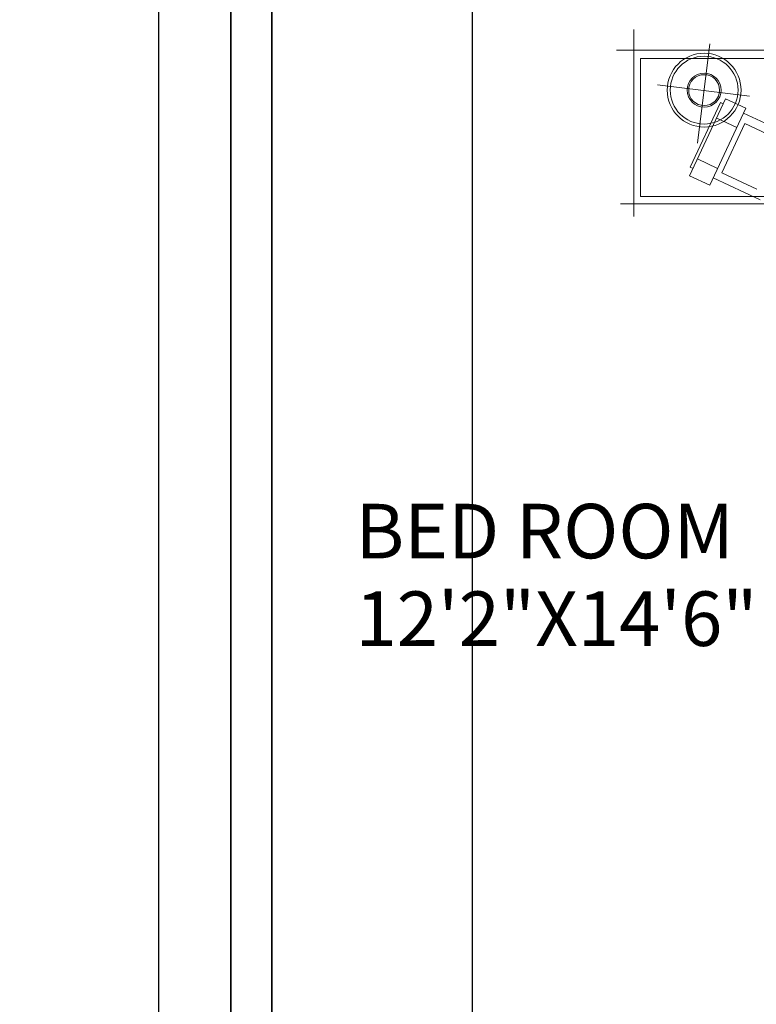
# Model space of a CAD drawing. Units: inches. Extents: x -438 to 102, y -60 to 1091.
# Tile 15 of 20: x -149 to -68, y 699 to 807. Entities that reach past the tile are written whole.
import ezdxf

# ---------------------------------------------------------------- set-up
doc = ezdxf.new("R2010")
doc.units = ezdxf.units.IN
doc.header["$MEASUREMENT"] = 0
doc.layers.add('A-ANNO-DIMS', color=217, linetype='Continuous', lineweight=18, true_color=0x93278f)
doc.layers.add('A-WALL', color=2, linetype='Continuous', lineweight=35, true_color=0xf1eb1f)
doc.layers.add('A-AREA-IDEN', color=4, linetype='Continuous', lineweight=18)
doc.layers.add('Furniture', color=7, linetype='Continuous', lineweight=15)
doc.styles.get("Standard").update_dxf_attribs({"font": 'arial.ttf'})
doc.dimstyles.get("Standard").update_dxf_attribs({"dimtxt": 8, "dimasz": 0.18, "dimexe": 0.18, "dimexo": 0.0625, "dimgap": 0.09, "dimtad": 0, "dimtih": 1, "dimtoh": 1, "dimdec": 4, "dimzin": 0, "dimdsep": 46, "dimlunit": 3, "dimtxsty": 'Standard', "dimcen": 0.09, "dimadec": 0, "dimazin": 0, "dimtfac": 1, "dimtdec": 4, "dimtofl": 0, "dimtmove": 0, "dimatfit": 3, "dimfxl": 1, "dimtolj": 1, "dimtzin": 0, "dimarcsym": 0})

# ---------------------------------------------------------------- blocks, each defined once
blk = doc.blocks.new('BED-DOUBLE-WITH-NIGHTSTANDS')
for p, q in [((-50.06, 0), (-50.06, -20.6)), ((-41.72, -1.6), (-43.05, -12.53)), ((-28.76, -2.28), (-51.98, -2.28)), ((-31.1, -3.21), (-49.32, -3.21)), ((-49.32, -3.21), (-49.32, -18.39)), ((-37.32, -7.35), (-47.47, -6.1)), ((-43.93, -16.11), (-39.96, -7.63)), ((-40.53, -8.03), (-43.86, -15.16)), ((-37.75, -8.67), (-41.72, -17.15)), ((-40.22, -8.18), (-40.53, -8.03)), ((-39.96, -7.63), (-37.75, -8.67)), ((-32.84, -11.63), (-38.01, -9.21)), ((-38.74, -10.79), (-40.95, -9.75)), ((-37.86, -10.36), (-40.39, -15.77)), ((-34, -12.16), (-37.86, -10.36)), ((-43.86, -15.16), (-43.55, -15.31)), ((-40.85, -15.29), (-43.06, -14.25)), ((-41.72, -17.15), (-43.93, -16.11)), ((-40.39, -15.77), (-36.53, -17.57)), ((-41.34, -16.34), (-36.18, -18.76)), ((-49.32, -18.39), (-31.1, -18.39)), ((-51.53, -19.21), (-28.85, -19.21))]:
    blk.add_line(p, q)
for radius in [4.06, 3.73, 1.87, 1.7]:
    blk.add_circle((-42.33, -6.68), radius)
blk = doc.blocks.new('*D37')
at = {"layer": 'A-ANNO-DIMS', "color": 0, "lineweight": -2, "transparency": 16777216}
for p, q in [((-179.8, 234.94), (-179.8, 1079.58)), ((-179.62, 1079.4), (-176.98, 1079.4)), ((-134.26, 1079.4), (-136.9, 1079.4)), ((-134.08, 234.94), (-134.08, 1079.58))]:
    blk.add_line(p, q, dxfattribs=at)
at = {"layer": 'A-ANNO-DIMS', "color": 0, "transparency": 16777216}
for points in [[(-179.62, 1079.43), (-179.62, 1079.37), (-179.8, 1079.4)], [(-134.26, 1079.43), (-134.26, 1079.37), (-134.08, 1079.4)]]:
    blk.add_solid(points, dxfattribs=at)
at = {"layer": 'Defpoints', "color": 0, "transparency": 16777216}
for p in [(-134.08, 1079.4), (-179.8, 234.88), (-134.08, 234.88)]:
    blk.add_point(p, dxfattribs=at)
at = {"layer": 'A-ANNO-DIMS', "color": 0, "transparency": 16777216, "insert": (-156.94, 1079.4), "char_height": 8, "attachment_point": 5}
blk.add_mtext('\\A1;3\'-9 1/2"', dxfattribs=at)
blk = doc.blocks.new('*D45')
at = {"layer": 'A-ANNO-DIMS', "color": 0, "lineweight": -2, "transparency": 16777216}
for p, q in [((-99.58, 615.92), (-99.58, 1079.58)), ((-99.4, 1079.4), (-59.27, 1079.4)), ((2.32, 1079.4), (-37.82, 1079.4)), ((2.5, 615.92), (2.5, 1079.58))]:
    blk.add_line(p, q, dxfattribs=at)
at = {"layer": 'A-ANNO-DIMS', "color": 0, "transparency": 16777216}
for points in [[(-99.4, 1079.43), (-99.4, 1079.37), (-99.58, 1079.4)], [(2.32, 1079.43), (2.32, 1079.37), (2.5, 1079.4)]]:
    blk.add_solid(points, dxfattribs=at)
at = {"layer": 'Defpoints', "color": 0, "transparency": 16777216}
for p in [(2.5, 1079.4), (-99.58, 615.86), (2.5, 615.86)]:
    blk.add_point(p, dxfattribs=at)
at = {"layer": 'A-ANNO-DIMS', "color": 0, "transparency": 16777216, "insert": (-48.54, 1079.4), "char_height": 8, "attachment_point": 5}
blk.add_mtext('\\A1;8\'-6"', dxfattribs=at)

msp = doc.modelspace()

# ---------------------------------------------------------------- linework, layer by layer
at = {"layer": 'A-WALL'}
for p, q in [((-126.14649, 665.49939), (-126.14649, 839.49939)), ((-121.64649, 665.49939), (-121.64649, 839.49939))]:
    msp.add_line(p, q, dxfattribs=at)

# ---------------------------------------------------------------- block references
at = {"layer": 'Furniture'}
msp.add_blockref('BED-DOUBLE-WITH-NIGHTSTANDS', (-31.753, 805.86269), dxfattribs=at)

# ---------------------------------------------------------------- texts
at = {"layer": 'A-AREA-IDEN'}
for s, p in [('BED ROOM', (-112.45711, 747.65778)), ('12\'2"X14\'6"', (-112.45711, 738.01931))]:
    msp.add_text(s, height=6, dxfattribs=at).set_placement(p)

# ---------------------------------------------------------------- dimensions: what is measured, and where the dimension line sits
at = {"layer": 'A-ANNO-DIMS'}
for base, p1, p2, picture, middle in [((-134.07948, 1079.39939), (-179.79585, 234.87846), (-134.07948, 234.87846), '*D37', (-156.93767, 1079.39939)), ((2.49567, 1079.39939), (-99.58389, 615.85716), (2.49567, 615.85716), '*D45', (-48.54411, 1079.39939))]:
    dim = msp.add_linear_dim(base=base, p1=p1, p2=p2, dimstyle='Standard', override={"dimdec": 1, "dimlfac": 1, "dimrnd": 0, "dimzin": 1, "dimdsep": 46, "dimlunit": 4, "dimfrac": 2}, dxfattribs=at)
    dim.commit()
    dim.dimension.update_dxf_attribs({"geometry": picture, "text_midpoint": middle})

doc.saveas('drawing.dxf')
